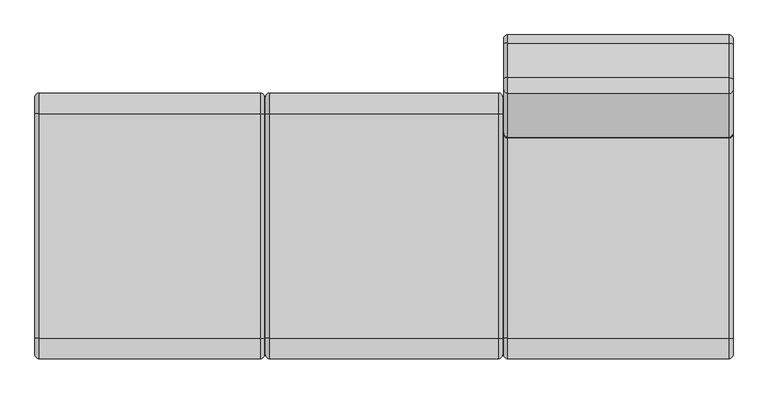
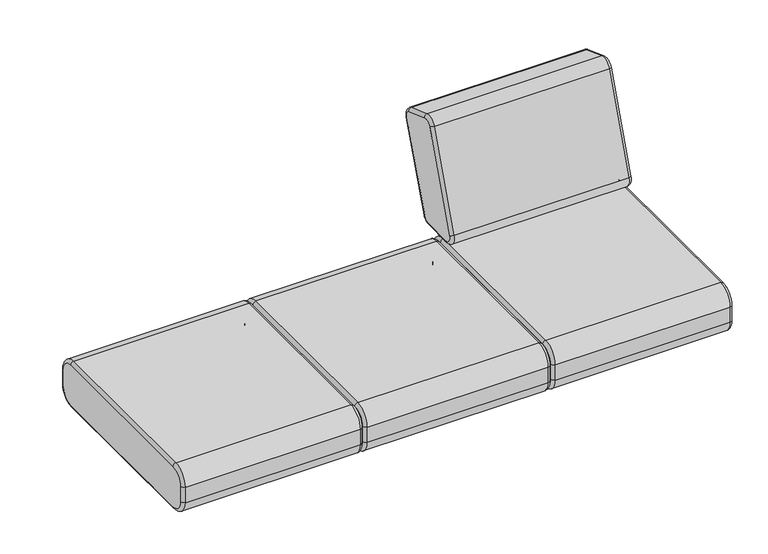
"""IFC4 building model written with IfcOpenShell, lengths in millimetres: furniture geometry."""

from ifc_helpers import new_model, si_unit, point, frame, origin, place, context, project, spatial, circle_curve, ellipse_curve, trimmed, source, transform, mapped, element, save
from ifc_brep_helpers import plane_surface, cylinder_surface, revolved_surface, advanced_brep


def furniture_29a9adb8(model_context):
    return source(origin(), model_context, "Body", "AdvancedBrep", [
        advanced_brep(
        [(-292.5, 542.7044583, 315.0), (-292.5, 582.7044583, 355.0), (-292.5, 582.7044583, 405.0), (-292.5, 542.7044583, 445.0), (-292.5, -5.0, 445.0), (-292.5, -45.0, 405.0), (-292.5, -45.0, 355.0), (-292.5, -5.0, 315.0), (-852.5, -5.0, 315.0), (-852.5, -45.0, 355.0), (-852.5, -45.0, 405.0), (-852.5, -5.0, 445.0), (-852.5, 542.7044583, 445.0), (-852.5, 582.7044583, 405.0), (-852.5, 582.7044583, 355.0), (-852.5, 542.7044583, 315.0), (-842.5, 592.7044583, 405.0), (-842.5, 542.7044583, 455.0), (-302.4999866, 542.7044583, 455.0), (-302.5, 592.7044583, 405.0), (-842.5, -5.0, 455.0), (-302.5, -5.0, 455.0), (-842.5, -55.0, 405.0), (-302.4999867, -55.0, 405.0), (-842.5, -55.0, 355.0), (-302.5, -55.0, 355.0), (-842.5, -5.0, 305.0), (-302.4999867, -5.0, 305.0), (-842.5, 542.7044583, 305.0), (-302.4999867, 542.7044583, 305.0), (-842.5, 592.7044583, 355.0), (-302.4999867, 592.7044583, 355.0)],
        [
            (0, 1, circle_curve(frame((-292.5, 542.7044583, 355.0), z_axis=(1.0, 0.0, 0.0), x_axis=(0.0, 0.0, -1.0)), 40.0)),
            (1, 2),
            (2, 3, circle_curve(frame((-292.5, 542.7044583, 405.0), z_axis=(1.0, 0.0, 0.0), x_axis=(0.0, 1.0, 0.0)), 40.0)),
            (3, 4),
            (4, 5, circle_curve(frame((-292.5, -5.0, 405.0), z_axis=(1.0, 0.0, 0.0), x_axis=(0.0, 0.0, 1.0)), 40.0)),
            (5, 6),
            (6, 7, circle_curve(frame((-292.5, -5.0, 355.0), z_axis=(1.0, 0.0, 0.0), x_axis=(0.0, -1.0, 0.0)), 40.0)),
            (7, 0),
            (8, 9, circle_curve(frame((-852.5, -5.0, 355.0), z_axis=(-1.0, 0.0, 0.0), x_axis=(0.0, 0.0, -1.0)), 40.0)),
            (9, 10),
            (10, 11, circle_curve(frame((-852.5, -5.0, 405.0), z_axis=(-1.0, 0.0, 0.0), x_axis=(0.0, -1.0, 0.0)), 40.0)),
            (11, 12),
            (12, 13, circle_curve(frame((-852.5, 542.7044583, 405.0), z_axis=(-1.0, 0.0, 0.0), x_axis=(0.0, 0.0, 1.0)), 40.0)),
            (13, 14),
            (14, 15, circle_curve(frame((-852.5, 542.7044583, 355.0), z_axis=(-1.0, 0.0, 0.0), x_axis=(0.0, 1.0, 0.0)), 40.0)),
            (15, 8),
            (16, 17, circle_curve(frame((-842.5, 542.7044583, 405.0), z_axis=(1.0, 0.0, 0.0), x_axis=(0.0, 1.0, 0.0)), 50.0)),
            (17, 18),
            (18, 19, circle_curve(frame((-302.5, 542.7044583, 405.0), z_axis=(-1.0, 0.0, 0.0), x_axis=(0.0, 1.0, 0.0)), 50.0)),
            (19, 16),
            (17, 20),
            (20, 21),
            (21, 18),
            (20, 22, circle_curve(frame((-842.5, -5.0, 405.0), z_axis=(1.0, 0.0, 0.0), x_axis=(0.0, 1.0, 0.0)), 50.0)),
            (22, 23),
            (23, 21, circle_curve(frame((-302.5, -5.0, 405.0), z_axis=(-1.0, 0.0, 0.0), x_axis=(0.0, 1.0, 0.0)), 50.0)),
            (22, 24),
            (24, 25),
            (25, 23),
            (24, 26, circle_curve(frame((-842.5, -5.0, 355.0), z_axis=(1.0, 0.0, 0.0), x_axis=(0.0, 1.0, 0.0)), 50.0)),
            (26, 27),
            (27, 25, circle_curve(frame((-302.5, -5.0, 355.0), z_axis=(-1.0, 0.0, 0.0), x_axis=(0.0, 1.0, 0.0)), 50.0)),
            (26, 28),
            (28, 29),
            (29, 27),
            (28, 30, circle_curve(frame((-842.5, 542.7044583, 355.0), z_axis=(1.0, 0.0, 0.0), x_axis=(0.0, 1.0, 0.0)), 50.0)),
            (30, 31),
            (31, 29, circle_curve(frame((-302.5, 542.7044583, 355.0), z_axis=(-1.0, 0.0, 0.0), x_axis=(0.0, 1.0, 0.0)), 50.0)),
            (30, 16),
            (19, 31),
            (24, 9, circle_curve(frame((-842.5, -45.0, 355.0), z_axis=(0.0, 0.0, -1.0), x_axis=(-1.0, 0.0, 0.0)), 10.0)),
            (8, 26, circle_curve(frame((-842.5, -5.0, 315.0), z_axis=(0.0, -1.0, 0.0), x_axis=(-1.0, 0.0, 0.0)), 10.0)),
            (22, 10, circle_curve(frame((-842.5, -45.0, 405.0), z_axis=(0.0, 0.0, -1.0), x_axis=(-1.0, 0.0, 0.0)), 10.0)),
            (20, 11, circle_curve(frame((-842.5, -5.0, 445.0), z_axis=(0.0, -1.0, 0.0), x_axis=(-1.0, 0.0, 0.0)), 10.0)),
            (17, 12, circle_curve(frame((-842.5, 542.7044583, 445.0), z_axis=(0.0, -1.0, 0.0), x_axis=(-1.0, 0.0, 0.0)), 10.0)),
            (16, 13, circle_curve(frame((-842.5, 582.7044583, 405.0), z_axis=(0.0, 0.0, 1.0), x_axis=(-1.0, 0.0, 0.0)), 10.0)),
            (30, 14, circle_curve(frame((-842.5, 582.7044583, 355.0), z_axis=(0.0, 0.0, 1.0), x_axis=(-1.0, 0.0, 0.0)), 10.0)),
            (28, 15, circle_curve(frame((-842.5, 542.7044583, 315.0), z_axis=(0.0, 1.0, 0.0), x_axis=(-1.0, 0.0, 0.0)), 10.0)),
            (31, 1, circle_curve(frame((-302.5, 582.7044583, 355.0), z_axis=(0.0, 0.0, -1.0), x_axis=(1.0, 0.0, 0.0)), 10.0)),
            (0, 29, circle_curve(frame((-302.5, 542.7044583, 315.0), z_axis=(0.0, 1.0, 0.0), x_axis=(1.0, 0.0, 0.0)), 10.0)),
            (19, 2, circle_curve(frame((-302.5, 582.7044583, 405.0), z_axis=(0.0, 0.0, -1.0), x_axis=(1.0, 0.0, 0.0)), 10.0)),
            (18, 3, circle_curve(frame((-302.5, 542.7044583, 445.0), z_axis=(0.0, 1.0, 0.0), x_axis=(1.0, 0.0, 0.0)), 10.0)),
            (21, 4, circle_curve(frame((-302.5, -5.0, 445.0), z_axis=(0.0, 1.0, 0.0), x_axis=(1.0, 0.0, 0.0)), 10.0)),
            (23, 5, circle_curve(frame((-302.5, -45.0, 405.0), z_axis=(0.0, 0.0, 1.0), x_axis=(1.0, 0.0, 0.0)), 10.0)),
            (25, 6, circle_curve(frame((-302.5, -45.0, 355.0), z_axis=(0.0, 0.0, 1.0), x_axis=(1.0, 0.0, 0.0)), 10.0)),
            (27, 7, circle_curve(frame((-302.5, -5.0, 315.0), z_axis=(0.0, -1.0, 0.0), x_axis=(1.0, 0.0, 0.0)), 10.0)),
        ],
        [
            plane_surface(frame((-292.5, 592.7044583, 405.0), z_axis=(1.0, 0.0, 0.0), x_axis=(0.0, 0.0, 1.0))),
            plane_surface(frame((-852.5, 592.7044583, 405.0), z_axis=(-1.0, 0.0, 0.0), x_axis=(0.0, 0.0, -1.0))),
            cylinder_surface(frame((-852.5, 542.7044583, 405.0), z_axis=(1.0, 0.0, 0.0), x_axis=(0.0, 1.0, 0.0)), 50.0),
            plane_surface(frame((-292.5, 542.7044583, 455.0), z_axis=(0.0, 0.0, 1.0), x_axis=(-1.0, 0.0, 0.0))),
            cylinder_surface(frame((-852.5, -5.0, 405.0), z_axis=(1.0, 0.0, 0.0), x_axis=(0.0, 1.0, 0.0)), 50.0),
            plane_surface(frame((-292.5, -55.0, 405.0), z_axis=(0.0, -1.0, 0.0), x_axis=(-1.0, 0.0, 0.0))),
            cylinder_surface(frame((-852.5, -5.0, 355.0), z_axis=(1.0, 0.0, 0.0), x_axis=(0.0, 1.0, 0.0)), 50.0),
            plane_surface(frame((-292.5, -5.0, 305.0), z_axis=(0.0, 0.0, -1.0), x_axis=(-1.0, 0.0, 0.0))),
            cylinder_surface(frame((-852.5, 542.7044583, 355.0), z_axis=(1.0, 0.0, 0.0), x_axis=(0.0, 1.0, 0.0)), 50.0),
            plane_surface(frame((-292.5, 592.7044583, 355.0), z_axis=(0.0, 1.0, 0.0), x_axis=(-1.0, 0.0, 0.0))),
            revolved_surface(trimmed(ellipse_curve(frame((-842.5, -5.0, 315.0), z_axis=(0.0, 1.0, 0.0), x_axis=(-1.0, 0.0, 0.0)), 10.0, 10.0), [point((-842.5, -5.0, 305.0))], [point((-852.5, -5.0, 315.0))], True, "CARTESIAN"), (-852.5, -5.0, 355.0), (-1.0, 0.0, 0.0)),
            cylinder_surface(frame((-842.5, -45.0, 355.0), z_axis=(0.0, 0.0, 1.0), x_axis=(-1.0, 0.0, 0.0)), 10.0),
            revolved_surface(trimmed(ellipse_curve(frame((-842.5, -45.0, 405.0), z_axis=(0.0, 0.0, -1.0), x_axis=(-1.0, 0.0, 0.0)), 10.0, 10.0), [point((-842.5, -55.0, 405.0))], [point((-852.5, -45.0, 405.0))], True, "CARTESIAN"), (-852.5, -5.0, 405.0), (-1.0, 0.0, 0.0)),
            cylinder_surface(frame((-842.5, -5.0, 445.0), z_axis=(0.0, 1.0, 0.0), x_axis=(-1.0, 0.0, 0.0)), 10.0),
            revolved_surface(trimmed(ellipse_curve(frame((-842.5, 542.7044583, 445.0), z_axis=(0.0, -1.0, 0.0), x_axis=(-1.0, 0.0, 0.0)), 10.0, 10.0), [point((-842.5, 542.7044583, 455.0))], [point((-852.5, 542.7044583, 445.0))], True, "CARTESIAN"), (-852.5, 542.7044583, 405.0), (-1.0, 0.0, 0.0)),
            cylinder_surface(frame((-842.5, 582.7044583, 405.0), z_axis=(0.0, 0.0, -1.0), x_axis=(-1.0, 0.0, 0.0)), 10.0),
            revolved_surface(trimmed(ellipse_curve(frame((-842.5, 582.7044583, 355.0), z_axis=(0.0, 0.0, 1.0), x_axis=(-1.0, 0.0, 0.0)), 10.0, 10.0), [point((-842.5, 592.7044583, 355.0))], [point((-852.5, 582.7044583, 355.0))], True, "CARTESIAN"), (-852.5, 542.7044583, 355.0), (-1.0, 0.0, 0.0)),
            cylinder_surface(frame((-842.5, 542.7044583, 315.0), z_axis=(0.0, -1.0, 0.0), x_axis=(-1.0, 0.0, 0.0)), 10.0),
            revolved_surface(trimmed(ellipse_curve(frame((-302.5, 542.7044583, 315.0), z_axis=(0.0, -1.0, 0.0), x_axis=(1.0, 0.0, 0.0)), 10.0, 10.0), [point((-302.5, 542.7044583, 305.0))], [point((-292.5, 542.7044583, 315.0))], True, "CARTESIAN"), (-292.5, 542.7044583, 355.0), (1.0, 0.0, 0.0)),
            cylinder_surface(frame((-302.5, 582.7044583, 355.0), z_axis=(0.0, 0.0, 1.0), x_axis=(1.0, 0.0, 0.0)), 10.0),
            revolved_surface(trimmed(ellipse_curve(frame((-302.5, 582.7044583, 405.0), z_axis=(0.0, 0.0, -1.0), x_axis=(1.0, 0.0, 0.0)), 10.0, 10.0), [point((-302.5, 592.7044583, 405.0))], [point((-292.5, 582.7044583, 405.0))], True, "CARTESIAN"), (-292.5, 542.7044583, 405.0), (1.0, 0.0, 0.0)),
            cylinder_surface(frame((-302.5, 542.7044583, 445.0), z_axis=(0.0, -1.0, 0.0), x_axis=(1.0, 0.0, 0.0)), 10.0),
            revolved_surface(trimmed(ellipse_curve(frame((-302.5, -5.0, 445.0), z_axis=(0.0, 1.0, 0.0), x_axis=(1.0, 0.0, 0.0)), 10.0, 10.0), [point((-302.5, -5.0, 455.0))], [point((-292.5, -5.0, 445.0))], True, "CARTESIAN"), (-292.5, -5.0, 405.0), (1.0, 0.0, 0.0)),
            cylinder_surface(frame((-302.5, -45.0, 405.0), z_axis=(0.0, 0.0, -1.0), x_axis=(1.0, 0.0, 0.0)), 10.0),
            revolved_surface(trimmed(ellipse_curve(frame((-302.5, -45.0, 355.0), z_axis=(0.0, 0.0, 1.0), x_axis=(1.0, 0.0, 0.0)), 10.0, 10.0), [point((-302.5, -55.0, 355.0))], [point((-292.5, -45.0, 355.0))], True, "CARTESIAN"), (-292.5, -5.0, 355.0), (1.0, 0.0, 0.0)),
            cylinder_surface(frame((-302.5, -5.0, 315.0), z_axis=(0.0, 1.0, 0.0), x_axis=(1.0, 0.0, 0.0)), 10.0),
        ],
        [
            (0, [[1, 2, 3, 4, 5, 6, 7, 8]]),
            (1, [[9, 10, 11, 12, 13, 14, 15, 16]]),
            (2, [[17, 18, 19, 20]]),
            (3, [[21, 22, 23, -18]]),
            (4, [[24, 25, 26, -22]]),
            (5, [[27, 28, 29, -25]]),
            (6, [[30, 31, 32, -28]]),
            (7, [[33, 34, 35, -31]]),
            (8, [[36, 37, 38, -34]]),
            (9, [[39, -20, 40, -37]]),
            (10, [[41, -9, 42, -30]]),
            (11, [[-41, -27, 43, -10]]),
            (12, [[-43, -24, 44, -11]]),
            (13, [[-44, -21, 45, -12]]),
            (14, [[-45, -17, 46, -13]]),
            (15, [[-46, -39, 47, -14]]),
            (16, [[-47, -36, 48, -15]]),
            (17, [[-42, -16, -48, -33]]),
            (18, [[49, -1, 50, -38]]),
            (19, [[-49, -40, 51, -2]]),
            (20, [[-51, -19, 52, -3]]),
            (21, [[-52, -23, 53, -4]]),
            (22, [[-53, -26, 54, -5]]),
            (23, [[-54, -29, 55, -6]]),
            (24, [[-55, -32, 56, -7]]),
            (25, [[-50, -8, -56, -35]]),
        ],
    ),
        advanced_brep(
        [(851.1853865, 609.5185405, 469.9348489), (851.1853865, 628.3736149, 483.1373142), (851.1853865, 723.5847628, 744.7277933), (851.1853865, 711.5923743, 770.4455535), (851.1853865, 627.0200384, 801.2273664), (851.1853865, 601.3022782, 789.2349779), (851.1853865, 494.8874666, 496.8626858), (851.1853865, 513.742541, 469.9348489), (291.1853865, 513.742541, 469.9348489), (291.1853865, 494.8874666, 496.8626858), (291.1853865, 601.3022782, 789.2349779), (291.1853865, 627.0200384, 801.2273664), (291.1853865, 711.5923743, 770.4455535), (291.1853865, 723.5847628, 744.7277933), (291.1853865, 628.3736149, 483.1373142), (291.1853865, 609.5185405, 469.9348489), (301.1853865, 630.4402399, 810.6242926), (301.1853865, 591.905352, 792.6551793), (841.1853984, 591.905352, 792.6551793), (841.1853865, 630.4402399, 810.6242926), (301.1853865, 485.4905403, 500.2828873), (841.1853865, 485.4905403, 500.2828873), (301.1853865, 513.742541, 459.9348489), (841.1853988, 513.742541, 459.9348489), (301.1853865, 609.5185405, 459.9348489), (841.1853987, 609.5185405, 459.9348489), (301.1853865, 637.7705411, 479.7171127), (841.1853987, 637.7705411, 479.7171127), (301.1853865, 732.9816891, 741.3075918), (841.1853865, 732.9816891, 741.3075918), (301.1853865, 715.0125757, 779.8424797), (841.1853984, 715.0125757, 779.8424797)],
        [
            (0, 1, circle_curve(frame((851.1853865, 609.5185405, 490.0), z_axis=(1.0, 0.0, 0.0), x_axis=(0.0, 0.0, -1.0)), 20.0651511)),
            (1, 2),
            (2, 3, circle_curve(frame((851.1853865, 704.7296884, 751.5904791), z_axis=(1.0, 0.0, 0.0), x_axis=(0.0, 0.9396926207859067, -0.3420201433256736)), 20.0651511)),
            (3, 4),
            (4, 5, circle_curve(frame((851.1853865, 620.1573526, 782.372292), z_axis=(1.0, 0.0, 0.0), x_axis=(0.0, 0.3420201433256753, 0.939692620785906)), 20.0651511)),
            (5, 6),
            (6, 7, circle_curve(frame((851.1853865, 513.742541, 490.0), z_axis=(1.0, 0.0, 0.0), x_axis=(0.0, -0.9396926207859095, 0.34202014332566555)), 20.0651511)),
            (7, 0),
            (8, 9, circle_curve(frame((291.1853865, 513.742541, 490.0), z_axis=(-1.0, 0.0, 0.0), x_axis=(0.0, 0.0, -1.0)), 20.0651511)),
            (9, 10),
            (10, 11, circle_curve(frame((291.1853865, 620.1573526, 782.372292), z_axis=(-1.0, 0.0, 0.0), x_axis=(0.0, -0.9396926207859101, 0.34202014332566405)), 20.0651511)),
            (11, 12),
            (12, 13, circle_curve(frame((291.1853865, 704.7296884, 751.5904791), z_axis=(-1.0, 0.0, 0.0), x_axis=(0.0, 0.34202014332566566, 0.9396926207859095)), 20.0651511)),
            (13, 14),
            (14, 15, circle_curve(frame((291.1853865, 609.5185405, 490.0), z_axis=(-1.0, 0.0, 0.0), x_axis=(0.0, 0.9396926207859108, -0.3420201433256623)), 20.0651511)),
            (15, 8),
            (16, 17, circle_curve(frame((301.1853865, 620.1573526, 782.372292), z_axis=(1.0, 0.0, 0.0), x_axis=(0.0, 1.0, 0.0)), 30.0651511)),
            (17, 18),
            (18, 19, circle_curve(frame((841.1853865, 620.1573526, 782.372292), z_axis=(-1.0, 0.0, 0.0), x_axis=(0.0, 1.0, 0.0)), 30.0651511)),
            (19, 16),
            (17, 20),
            (20, 21),
            (21, 18),
            (20, 22, circle_curve(frame((301.1853865, 513.742541, 490.0), z_axis=(1.0, 0.0, 0.0), x_axis=(0.0, 1.0, 0.0)), 30.0651511)),
            (22, 23),
            (23, 21, circle_curve(frame((841.1853865, 513.742541, 490.0), z_axis=(-1.0, 0.0, 0.0), x_axis=(0.0, 1.0, 0.0)), 30.0651511)),
            (22, 24),
            (24, 25),
            (25, 23),
            (24, 26, circle_curve(frame((301.1853865, 609.5185405, 490.0), z_axis=(1.0, 0.0, 0.0), x_axis=(0.0, 1.0, 0.0)), 30.0651511)),
            (26, 27),
            (27, 25, circle_curve(frame((841.1853865, 609.5185405, 490.0), z_axis=(-1.0, 0.0, 0.0), x_axis=(0.0, 1.0, 0.0)), 30.0651511)),
            (26, 28),
            (28, 29),
            (29, 27),
            (28, 30, circle_curve(frame((301.1853865, 704.7296884, 751.5904791), z_axis=(1.0, 0.0, 0.0), x_axis=(0.0, 1.0, 0.0)), 30.0651511)),
            (30, 31),
            (31, 29, circle_curve(frame((841.1853865, 704.7296884, 751.5904791), z_axis=(-1.0, 0.0, 0.0), x_axis=(0.0, 1.0, 0.0)), 30.0651511)),
            (30, 16),
            (19, 31),
            (20, 9, circle_curve(frame((301.1853865, 494.8874666, 496.8626858), z_axis=(0.0, -0.34202014332566616, -0.9396926207859093), x_axis=(-1.0, 0.0, 0.0)), 10.0)),
            (8, 22, circle_curve(frame((301.1853865, 513.742541, 469.9348489), z_axis=(0.0, -1.0, 0.0), x_axis=(-1.0, 0.0, 0.0)), 10.0)),
            (17, 10, circle_curve(frame((301.1853865, 601.3022782, 789.2349779), z_axis=(0.0, -0.3420201433256583, -0.9396926207859122), x_axis=(-1.0, 0.0, 0.0)), 10.0)),
            (16, 11, circle_curve(frame((301.1853865, 627.0200384, 801.2273664), z_axis=(0.0, -0.9396926207859073, 0.34202014332567154), x_axis=(-1.0, 0.0, 0.0)), 10.0)),
            (30, 12, circle_curve(frame((301.1853865, 711.5923743, 770.4455535), z_axis=(0.0, -0.9396926207859225, 0.34202014332562997), x_axis=(-1.0, 0.0, 0.0)), 10.0)),
            (28, 13, circle_curve(frame((301.1853865, 723.5847628, 744.7277933), z_axis=(0.0, 0.34202014332567504, 0.9396926207859061), x_axis=(-1.0, 0.0, 0.0)), 10.0)),
            (26, 14, circle_curve(frame((301.1853865, 628.3736149, 483.1373142), z_axis=(0.0, 0.34202014332565633, 0.939692620785913), x_axis=(-1.0, 0.0, 0.0)), 10.0)),
            (24, 15, circle_curve(frame((301.1853865, 609.5185405, 469.9348489), z_axis=(0.0, 0.9999999999999999, 0.0), x_axis=(-1.0, 0.0, 0.0)), 10.0)),
            (27, 1, circle_curve(frame((841.1853865, 628.3736149, 483.1373142), z_axis=(0.0, -0.3420201433256674, -0.9396926207859089), x_axis=(1.0, 0.0, 0.0)), 10.0)),
            (0, 25, circle_curve(frame((841.1853865, 609.5185405, 469.9348489), z_axis=(0.0, 1.0, 0.0), x_axis=(1.0, 0.0, 0.0)), 10.0)),
            (29, 2, circle_curve(frame((841.1853865, 723.5847628, 744.7277933), z_axis=(0.0, -0.34202014332565644, -0.9396926207859129), x_axis=(1.0, 0.0, 0.0)), 10.0)),
            (31, 3, circle_curve(frame((841.1853865, 711.5923743, 770.4455535), z_axis=(0.0, 0.9396926207859082, -0.3420201433256694), x_axis=(1.0, 0.0, 0.0)), 10.0)),
            (19, 4, circle_curve(frame((841.1853865, 627.0200384, 801.2273664), z_axis=(0.0, 0.9396926207859224, -0.3420201433256302), x_axis=(1.0, 0.0, 0.0)), 10.0)),
            (18, 5, circle_curve(frame((841.1853865, 601.3022782, 789.2349779), z_axis=(0.0, 0.34202014332566893, 0.9396926207859083), x_axis=(1.0, 0.0, 0.0)), 10.0)),
            (21, 6, circle_curve(frame((841.1853865, 494.8874666, 496.8626858), z_axis=(0.0, 0.3420201433256585, 0.9396926207859122), x_axis=(1.0, 0.0, 0.0)), 10.0)),
            (23, 7, circle_curve(frame((841.1853865, 513.742541, 469.9348489), z_axis=(0.0, -1.0, 0.0), x_axis=(1.0, 0.0, 0.0)), 10.0)),
        ],
        [
            plane_surface(frame((851.1853865, 650.2225036, 782.372292), z_axis=(1.0, 0.0, 0.0), x_axis=(0.0, 0.0, 1.0))),
            plane_surface(frame((291.1853865, 650.2225036, 782.372292), z_axis=(-1.0, 0.0, 0.0), x_axis=(0.0, 0.0, -1.0))),
            cylinder_surface(frame((291.1853865, 620.1573526, 782.372292), z_axis=(1.0, 0.0, 0.0), x_axis=(0.0, 1.0, 0.0)), 30.0651511),
            plane_surface(frame((851.1853865, 591.905352, 792.6551793), z_axis=(0.0, -0.9396926207859123, 0.3420201433256582), x_axis=(-1.0, 0.0, 0.0))),
            cylinder_surface(frame((291.1853865, 513.742541, 490.0), z_axis=(1.0, 0.0, 0.0), x_axis=(0.0, 1.0, 0.0)), 30.0651511),
            plane_surface(frame((851.1853865, 513.742541, 459.9348489), z_axis=(0.0, 0.0, -1.0), x_axis=(-1.0, 0.0, 0.0))),
            cylinder_surface(frame((291.1853865, 609.5185405, 490.0), z_axis=(1.0, 0.0, 0.0), x_axis=(0.0, 1.0, 0.0)), 30.0651511),
            plane_surface(frame((851.1853865, 637.7705411, 479.7171127), z_axis=(0.0, 0.9396926207859131, -0.3420201433256561), x_axis=(-1.0, 0.0, 0.0))),
            cylinder_surface(frame((291.1853865, 704.7296884, 751.5904791), z_axis=(1.0, 0.0, 0.0), x_axis=(0.0, 1.0, 0.0)), 30.0651511),
            plane_surface(frame((851.1853865, 715.0125757, 779.8424797), z_axis=(0.0, 0.34202014332562986, 0.9396926207859226), x_axis=(-1.0, 0.0, 0.0))),
            revolved_surface(trimmed(ellipse_curve(frame((301.1853865, 513.742541, 469.9348489), z_axis=(0.0, 1.0, 0.0), x_axis=(-1.0, 0.0, 0.0)), 10.0, 10.0), [point((301.1853865, 513.742541, 459.9348489))], [point((291.1853865, 513.742541, 469.9348489))], True, "CARTESIAN"), (291.1853865, 513.742541, 490.0), (-1.0, 0.0, 0.0)),
            cylinder_surface(frame((301.1853865, 494.8874666, 496.8626858), z_axis=(0.0, 0.3420201433256583, 0.9396926207859122), x_axis=(-1.0, 0.0, 0.0)), 10.0),
            revolved_surface(trimmed(ellipse_curve(frame((301.1853865, 601.3022782, 789.2349779), z_axis=(0.0, -0.3420201433256641, -0.9396926207859101), x_axis=(-1.0, 0.0, 0.0)), 10.0, 10.0), [point((301.1853865, 591.905352, 792.6551793))], [point((291.1853865, 601.3022782, 789.2349779))], True, "CARTESIAN"), (291.1853865, 620.1573526, 782.372292), (-1.0, 0.0, 0.0)),
            cylinder_surface(frame((301.1853865, 627.0200384, 801.2273664), z_axis=(0.0, 0.9396926207859225, -0.34202014332562997), x_axis=(-1.0, 0.0, 0.0)), 10.0),
            revolved_surface(trimmed(ellipse_curve(frame((301.1853865, 711.5923743, 770.4455535), z_axis=(0.0, -0.9396926207859094, 0.34202014332566594), x_axis=(-1.0, 0.0, 0.0)), 10.0, 10.0), [point((301.1853865, 715.0125757, 779.8424797))], [point((291.1853865, 711.5923743, 770.4455535))], True, "CARTESIAN"), (291.1853865, 704.7296884, 751.5904791), (-1.0, 0.0, 0.0)),
            cylinder_surface(frame((301.1853865, 723.5847628, 744.7277933), z_axis=(0.0, -0.34202014332565633, -0.939692620785913), x_axis=(-1.0, 0.0, 0.0)), 10.0),
            revolved_surface(trimmed(ellipse_curve(frame((301.1853865, 628.3736149, 483.1373142), z_axis=(0.0, 0.3420201433256624, 0.9396926207859108), x_axis=(-1.0, 0.0, 0.0)), 10.0, 10.0), [point((301.1853865, 637.7705411, 479.7171127))], [point((291.1853865, 628.3736149, 483.1373142))], True, "CARTESIAN"), (291.1853865, 609.5185405, 490.0), (-1.0, 0.0, 0.0)),
            cylinder_surface(frame((301.1853865, 609.5185405, 469.9348489), z_axis=(0.0, -1.0, 0.0), x_axis=(-1.0, 0.0, 0.0)), 10.0),
            revolved_surface(trimmed(ellipse_curve(frame((841.1853865, 609.5185405, 469.9348489), z_axis=(0.0, -1.0, 0.0), x_axis=(1.0, 0.0, 0.0)), 10.0, 10.0), [point((841.1853865, 609.5185405, 459.9348489))], [point((851.1853865, 609.5185405, 469.9348489))], True, "CARTESIAN"), (851.1853865, 609.5185405, 490.0), (1.0, 0.0, 0.0)),
            cylinder_surface(frame((841.1853865, 628.3736149, 483.1373142), z_axis=(0.0, 0.34202014332565644, 0.9396926207859129), x_axis=(1.0, 0.0, 0.0)), 10.0),
            revolved_surface(trimmed(ellipse_curve(frame((841.1853865, 723.5847628, 744.7277933), z_axis=(0.0, -0.34202014332567393, -0.9396926207859065), x_axis=(1.0, 0.0, 0.0)), 10.0, 10.0), [point((841.1853865, 732.9816891, 741.3075918))], [point((851.1853865, 723.5847628, 744.7277933))], True, "CARTESIAN"), (851.1853865, 704.7296884, 751.5904791), (1.0, 0.0, 0.0)),
            cylinder_surface(frame((841.1853865, 711.5923743, 770.4455535), z_axis=(0.0, -0.9396926207859224, 0.3420201433256302), x_axis=(1.0, 0.0, 0.0)), 10.0),
            revolved_surface(trimmed(ellipse_curve(frame((841.1853865, 627.0200384, 801.2273664), z_axis=(0.0, 0.9396926207859059, -0.3420201433256756), x_axis=(1.0, 0.0, 0.0)), 10.0, 10.0), [point((841.1853865, 630.4402399, 810.6242926))], [point((851.1853865, 627.0200384, 801.2273664))], True, "CARTESIAN"), (851.1853865, 620.1573526, 782.372292), (1.0, 0.0, 0.0)),
            cylinder_surface(frame((841.1853865, 601.3022782, 789.2349779), z_axis=(0.0, -0.3420201433256585, -0.9396926207859122), x_axis=(1.0, 0.0, 0.0)), 10.0),
            revolved_surface(trimmed(ellipse_curve(frame((841.1853865, 494.8874666, 496.8626858), z_axis=(0.0, 0.34202014332566594, 0.9396926207859094), x_axis=(1.0, 0.0, 0.0)), 10.0, 10.0), [point((841.1853865, 485.4905403, 500.2828873))], [point((851.1853865, 494.8874666, 496.8626858))], True, "CARTESIAN"), (851.1853865, 513.742541, 490.0), (1.0, 0.0, 0.0)),
            cylinder_surface(frame((841.1853865, 513.742541, 469.9348489), z_axis=(0.0, 1.0, 0.0), x_axis=(1.0, 0.0, 0.0)), 10.0),
        ],
        [
            (0, [[1, 2, 3, 4, 5, 6, 7, 8]]),
            (1, [[9, 10, 11, 12, 13, 14, 15, 16]]),
            (2, [[17, 18, 19, 20]]),
            (3, [[21, 22, 23, -18]]),
            (4, [[24, 25, 26, -22]]),
            (5, [[27, 28, 29, -25]]),
            (6, [[30, 31, 32, -28]]),
            (7, [[33, 34, 35, -31]]),
            (8, [[36, 37, 38, -34]]),
            (9, [[39, -20, 40, -37]]),
            (10, [[41, -9, 42, -24]]),
            (11, [[-41, -21, 43, -10]]),
            (12, [[-43, -17, 44, -11]]),
            (13, [[-44, -39, 45, -12]]),
            (14, [[-45, -36, 46, -13]]),
            (15, [[-46, -33, 47, -14]]),
            (16, [[-47, -30, 48, -15]]),
            (17, [[-42, -16, -48, -27]]),
            (18, [[49, -1, 50, -32]]),
            (19, [[-49, -35, 51, -2]]),
            (20, [[-51, -38, 52, -3]]),
            (21, [[-52, -40, 53, -4]]),
            (22, [[-53, -19, 54, -5]]),
            (23, [[-54, -23, 55, -6]]),
            (24, [[-55, -26, 56, -7]]),
            (25, [[-50, -8, -56, -29]]),
        ],
    ),
        advanced_brep(
        [(851.1853865, 542.7044583, 315.0), (851.1853865, 582.7044583, 355.0), (851.1853865, 582.7044583, 405.0), (851.1853865, 542.7044583, 445.0), (851.1853865, -5.0, 445.0), (851.1853865, -45.0, 405.0), (851.1853865, -45.0, 355.0), (851.1853865, -5.0, 315.0), (291.1853865, -5.0, 315.0), (291.1853865, -45.0, 355.0), (291.1853865, -45.0, 405.0), (291.1853865, -5.0, 445.0), (291.1853865, 542.7044583, 445.0), (291.1853865, 582.7044583, 405.0), (291.1853865, 582.7044583, 355.0), (291.1853865, 542.7044583, 315.0), (301.1853865, 592.7044583, 405.0), (301.1853865, 542.7044583, 455.0), (841.1854, 542.7044583, 455.0), (841.1853865, 592.7044583, 405.0), (301.1853865, -5.0, 455.0), (841.1853865, -5.0, 455.0), (301.1853865, -55.0, 405.0), (841.1854, -55.0, 405.0), (301.1853865, -55.0, 355.0), (841.1853865, -55.0, 355.0), (301.1853865, -5.0, 305.0), (841.1853999, -5.0, 305.0), (301.1853865, 542.7044583, 305.0), (841.1854, 542.7044583, 305.0), (301.1853865, 592.7044583, 355.0), (841.1854, 592.7044583, 355.0)],
        [
            (0, 1, circle_curve(frame((851.1853865, 542.7044583, 355.0), z_axis=(1.0, 0.0, 0.0), x_axis=(0.0, 0.0, -1.0)), 40.0)),
            (1, 2),
            (2, 3, circle_curve(frame((851.1853865, 542.7044583, 405.0), z_axis=(1.0, 0.0, 0.0), x_axis=(0.0, 1.0, 0.0)), 40.0)),
            (3, 4),
            (4, 5, circle_curve(frame((851.1853865, -5.0, 405.0), z_axis=(1.0, 0.0, 0.0), x_axis=(0.0, 0.0, 1.0)), 40.0)),
            (5, 6),
            (6, 7, circle_curve(frame((851.1853865, -5.0, 355.0), z_axis=(1.0, 0.0, 0.0), x_axis=(0.0, -1.0, 0.0)), 40.0)),
            (7, 0),
            (8, 9, circle_curve(frame((291.1853865, -5.0, 355.0), z_axis=(-1.0, 0.0, 0.0), x_axis=(0.0, 0.0, -1.0)), 40.0)),
            (9, 10),
            (10, 11, circle_curve(frame((291.1853865, -5.0, 405.0), z_axis=(-1.0, 0.0, 0.0), x_axis=(0.0, -1.0, 0.0)), 40.0)),
            (11, 12),
            (12, 13, circle_curve(frame((291.1853865, 542.7044583, 405.0), z_axis=(-1.0, 0.0, 0.0), x_axis=(0.0, 0.0, 1.0)), 40.0)),
            (13, 14),
            (14, 15, circle_curve(frame((291.1853865, 542.7044583, 355.0), z_axis=(-1.0, 0.0, 0.0), x_axis=(0.0, 1.0, 0.0)), 40.0)),
            (15, 8),
            (16, 17, circle_curve(frame((301.1853865, 542.7044583, 405.0), z_axis=(1.0, 0.0, 0.0), x_axis=(0.0, 1.0, 0.0)), 50.0)),
            (17, 18),
            (18, 19, circle_curve(frame((841.1853865, 542.7044583, 405.0), z_axis=(-1.0, 0.0, 0.0), x_axis=(0.0, 1.0, 0.0)), 50.0)),
            (19, 16),
            (17, 20),
            (20, 21),
            (21, 18),
            (20, 22, circle_curve(frame((301.1853865, -5.0, 405.0), z_axis=(1.0, 0.0, 0.0), x_axis=(0.0, 1.0, 0.0)), 50.0)),
            (22, 23),
            (23, 21, circle_curve(frame((841.1853865, -5.0, 405.0), z_axis=(-1.0, 0.0, 0.0), x_axis=(0.0, 1.0, 0.0)), 50.0)),
            (22, 24),
            (24, 25),
            (25, 23),
            (24, 26, circle_curve(frame((301.1853865, -5.0, 355.0), z_axis=(1.0, 0.0, 0.0), x_axis=(0.0, 1.0, 0.0)), 50.0)),
            (26, 27),
            (27, 25, circle_curve(frame((841.1853865, -5.0, 355.0), z_axis=(-1.0, 0.0, 0.0), x_axis=(0.0, 1.0, 0.0)), 50.0)),
            (26, 28),
            (28, 29),
            (29, 27),
            (28, 30, circle_curve(frame((301.1853865, 542.7044583, 355.0), z_axis=(1.0, 0.0, 0.0), x_axis=(0.0, 1.0, 0.0)), 50.0)),
            (30, 31),
            (31, 29, circle_curve(frame((841.1853865, 542.7044583, 355.0), z_axis=(-1.0, 0.0, 0.0), x_axis=(0.0, 1.0, 0.0)), 50.0)),
            (30, 16),
            (19, 31),
            (24, 9, circle_curve(frame((301.1853865, -45.0, 355.0), z_axis=(0.0, 0.0, -1.0), x_axis=(-1.0, 0.0, 0.0)), 10.0)),
            (8, 26, circle_curve(frame((301.1853865, -5.0, 315.0), z_axis=(0.0, -1.0, 0.0), x_axis=(-1.0, 0.0, 0.0)), 10.0)),
            (22, 10, circle_curve(frame((301.1853865, -45.0, 405.0), z_axis=(0.0, 0.0, -1.0), x_axis=(-1.0, 0.0, 0.0)), 10.0)),
            (20, 11, circle_curve(frame((301.1853865, -5.0, 445.0), z_axis=(0.0, -1.0, 0.0), x_axis=(-1.0, 0.0, 0.0)), 10.0)),
            (17, 12, circle_curve(frame((301.1853865, 542.7044583, 445.0), z_axis=(0.0, -1.0, 0.0), x_axis=(-1.0, 0.0, 0.0)), 10.0)),
            (16, 13, circle_curve(frame((301.1853865, 582.7044583, 405.0), z_axis=(0.0, 0.0, 1.0), x_axis=(-1.0, 0.0, 0.0)), 10.0)),
            (30, 14, circle_curve(frame((301.1853865, 582.7044583, 355.0), z_axis=(0.0, 0.0, 1.0), x_axis=(-1.0, 0.0, 0.0)), 10.0)),
            (28, 15, circle_curve(frame((301.1853865, 542.7044583, 315.0), z_axis=(0.0, 1.0, 0.0), x_axis=(-1.0, 0.0, 0.0)), 10.0)),
            (31, 1, circle_curve(frame((841.1853865, 582.7044583, 355.0), z_axis=(0.0, 0.0, -1.0), x_axis=(1.0, 0.0, 0.0)), 10.0)),
            (0, 29, circle_curve(frame((841.1853865, 542.7044583, 315.0), z_axis=(0.0, 1.0, 0.0), x_axis=(1.0, 0.0, 0.0)), 10.0)),
            (19, 2, circle_curve(frame((841.1853865, 582.7044583, 405.0), z_axis=(0.0, 0.0, -1.0), x_axis=(1.0, 0.0, 0.0)), 10.0)),
            (18, 3, circle_curve(frame((841.1853865, 542.7044583, 445.0), z_axis=(0.0, 1.0, 0.0), x_axis=(1.0, 0.0, 0.0)), 10.0)),
            (21, 4, circle_curve(frame((841.1853865, -5.0, 445.0), z_axis=(0.0, 1.0, 0.0), x_axis=(1.0, 0.0, 0.0)), 10.0)),
            (23, 5, circle_curve(frame((841.1853865, -45.0, 405.0), z_axis=(0.0, 0.0, 1.0), x_axis=(1.0, 0.0, 0.0)), 10.0)),
            (25, 6, circle_curve(frame((841.1853865, -45.0, 355.0), z_axis=(0.0, 0.0, 1.0), x_axis=(1.0, 0.0, 0.0)), 10.0)),
            (27, 7, circle_curve(frame((841.1853865, -5.0, 315.0), z_axis=(0.0, -1.0, 0.0), x_axis=(1.0, 0.0, 0.0)), 10.0)),
        ],
        [
            plane_surface(frame((851.1853865, 592.7044583, 405.0), z_axis=(1.0, 0.0, 0.0), x_axis=(0.0, 0.0, 1.0))),
            plane_surface(frame((291.1853865, 592.7044583, 405.0), z_axis=(-1.0, 0.0, 0.0), x_axis=(0.0, 0.0, -1.0))),
            cylinder_surface(frame((291.1853865, 542.7044583, 405.0), z_axis=(1.0, 0.0, 0.0), x_axis=(0.0, 1.0, 0.0)), 50.0),
            plane_surface(frame((851.1853865, 542.7044583, 455.0), z_axis=(0.0, 0.0, 1.0), x_axis=(-1.0, 0.0, 0.0))),
            cylinder_surface(frame((291.1853865, -5.0, 405.0), z_axis=(1.0, 0.0, 0.0), x_axis=(0.0, 1.0, 0.0)), 50.0),
            plane_surface(frame((851.1853865, -55.0, 405.0), z_axis=(0.0, -1.0, 0.0), x_axis=(-1.0, 0.0, 0.0))),
            cylinder_surface(frame((291.1853865, -5.0, 355.0), z_axis=(1.0, 0.0, 0.0), x_axis=(0.0, 1.0, 0.0)), 50.0),
            plane_surface(frame((851.1853865, -5.0, 305.0), z_axis=(0.0, 0.0, -1.0), x_axis=(-1.0, 0.0, 0.0))),
            cylinder_surface(frame((291.1853865, 542.7044583, 355.0), z_axis=(1.0, 0.0, 0.0), x_axis=(0.0, 1.0, 0.0)), 50.0),
            plane_surface(frame((851.1853865, 592.7044583, 355.0), z_axis=(0.0, 1.0, 0.0), x_axis=(-1.0, 0.0, 0.0))),
            revolved_surface(trimmed(ellipse_curve(frame((301.1853865, -5.0, 315.0), z_axis=(0.0, 1.0, 0.0), x_axis=(-1.0, 0.0, 0.0)), 10.0, 10.0), [point((301.1853865, -5.0, 305.0))], [point((291.1853865, -5.0, 315.0))], True, "CARTESIAN"), (291.1853865, -5.0, 355.0), (-1.0, 0.0, 0.0)),
            cylinder_surface(frame((301.1853865, -45.0, 355.0), z_axis=(0.0, 0.0, 1.0), x_axis=(-1.0, 0.0, 0.0)), 10.0),
            revolved_surface(trimmed(ellipse_curve(frame((301.1853865, -45.0, 405.0), z_axis=(0.0, 0.0, -1.0), x_axis=(-1.0, 0.0, 0.0)), 10.0, 10.0), [point((301.1853865, -55.0, 405.0))], [point((291.1853865, -45.0, 405.0))], True, "CARTESIAN"), (291.1853865, -5.0, 405.0), (-1.0, 0.0, 0.0)),
            cylinder_surface(frame((301.1853865, -5.0, 445.0), z_axis=(0.0, 1.0, 0.0), x_axis=(-1.0, 0.0, 0.0)), 10.0),
            revolved_surface(trimmed(ellipse_curve(frame((301.1853865, 542.7044583, 445.0), z_axis=(0.0, -1.0, 0.0), x_axis=(-1.0, 0.0, 0.0)), 10.0, 10.0), [point((301.1853865, 542.7044583, 455.0))], [point((291.1853865, 542.7044583, 445.0))], True, "CARTESIAN"), (291.1853865, 542.7044583, 405.0), (-1.0, 0.0, 0.0)),
            cylinder_surface(frame((301.1853865, 582.7044583, 405.0), z_axis=(0.0, 0.0, -1.0), x_axis=(-1.0, 0.0, 0.0)), 10.0),
            revolved_surface(trimmed(ellipse_curve(frame((301.1853865, 582.7044583, 355.0), z_axis=(0.0, 0.0, 1.0), x_axis=(-1.0, 0.0, 0.0)), 10.0, 10.0), [point((301.1853865, 592.7044583, 355.0))], [point((291.1853865, 582.7044583, 355.0))], True, "CARTESIAN"), (291.1853865, 542.7044583, 355.0), (-1.0, 0.0, 0.0)),
            cylinder_surface(frame((301.1853865, 542.7044583, 315.0), z_axis=(0.0, -1.0, 0.0), x_axis=(-1.0, 0.0, 0.0)), 10.0),
            revolved_surface(trimmed(ellipse_curve(frame((841.1853865, 542.7044583, 315.0), z_axis=(0.0, -1.0, 0.0), x_axis=(1.0, 0.0, 0.0)), 10.0, 10.0), [point((841.1853865, 542.7044583, 305.0))], [point((851.1853865, 542.7044583, 315.0))], True, "CARTESIAN"), (851.1853865, 542.7044583, 355.0), (1.0, 0.0, 0.0)),
            cylinder_surface(frame((841.1853865, 582.7044583, 355.0), z_axis=(0.0, 0.0, 1.0), x_axis=(1.0, 0.0, 0.0)), 10.0),
            revolved_surface(trimmed(ellipse_curve(frame((841.1853865, 582.7044583, 405.0), z_axis=(0.0, 0.0, -1.0), x_axis=(1.0, 0.0, 0.0)), 10.0, 10.0), [point((841.1853865, 592.7044583, 405.0))], [point((851.1853865, 582.7044583, 405.0))], True, "CARTESIAN"), (851.1853865, 542.7044583, 405.0), (1.0, 0.0, 0.0)),
            cylinder_surface(frame((841.1853865, 542.7044583, 445.0), z_axis=(0.0, -1.0, 0.0), x_axis=(1.0, 0.0, 0.0)), 10.0),
            revolved_surface(trimmed(ellipse_curve(frame((841.1853865, -5.0, 445.0), z_axis=(0.0, 1.0, 0.0), x_axis=(1.0, 0.0, 0.0)), 10.0, 10.0), [point((841.1853865, -5.0, 455.0))], [point((851.1853865, -5.0, 445.0))], True, "CARTESIAN"), (851.1853865, -5.0, 405.0), (1.0, 0.0, 0.0)),
            cylinder_surface(frame((841.1853865, -45.0, 405.0), z_axis=(0.0, 0.0, -1.0), x_axis=(1.0, 0.0, 0.0)), 10.0),
            revolved_surface(trimmed(ellipse_curve(frame((841.1853865, -45.0, 355.0), z_axis=(0.0, 0.0, 1.0), x_axis=(1.0, 0.0, 0.0)), 10.0, 10.0), [point((841.1853865, -55.0, 355.0))], [point((851.1853865, -45.0, 355.0))], True, "CARTESIAN"), (851.1853865, -5.0, 355.0), (1.0, 0.0, 0.0)),
            cylinder_surface(frame((841.1853865, -5.0, 315.0), z_axis=(0.0, 1.0, 0.0), x_axis=(1.0, 0.0, 0.0)), 10.0),
        ],
        [
            (0, [[1, 2, 3, 4, 5, 6, 7, 8]]),
            (1, [[9, 10, 11, 12, 13, 14, 15, 16]]),
            (2, [[17, 18, 19, 20]]),
            (3, [[21, 22, 23, -18]]),
            (4, [[24, 25, 26, -22]]),
            (5, [[27, 28, 29, -25]]),
            (6, [[30, 31, 32, -28]]),
            (7, [[33, 34, 35, -31]]),
            (8, [[36, 37, 38, -34]]),
            (9, [[39, -20, 40, -37]]),
            (10, [[41, -9, 42, -30]]),
            (11, [[-41, -27, 43, -10]]),
            (12, [[-43, -24, 44, -11]]),
            (13, [[-44, -21, 45, -12]]),
            (14, [[-45, -17, 46, -13]]),
            (15, [[-46, -39, 47, -14]]),
            (16, [[-47, -36, 48, -15]]),
            (17, [[-42, -16, -48, -33]]),
            (18, [[49, -1, 50, -38]]),
            (19, [[-49, -40, 51, -2]]),
            (20, [[-51, -19, 52, -3]]),
            (21, [[-52, -23, 53, -4]]),
            (22, [[-53, -26, 54, -5]]),
            (23, [[-54, -29, 55, -6]]),
            (24, [[-55, -32, 56, -7]]),
            (25, [[-50, -8, -56, -35]]),
        ],
    ),
        advanced_brep(
        [(288.5853906, 542.7044583, 315.0), (288.5853906, 582.7044583, 355.0), (288.5853906, 582.7044583, 405.0), (288.5853906, 542.7044583, 445.0), (288.5853906, -5.0, 445.0), (288.5853906, -45.0, 405.0), (288.5853906, -45.0, 355.0), (288.5853906, -5.0, 315.0), (-290.0, 542.7044583, 445.0), (-290.0, 582.7044583, 405.0), (-290.0, 582.7044583, 355.0), (-290.0, 542.7044583, 315.0), (-290.0, -5.0, 315.0), (-290.0, -45.0, 355.0), (-290.0, -45.0, 405.0), (-290.0, -5.0, 445.0), (-280.0, 592.7044583, 405.0), (-280.0, 542.7044583, 455.0), (278.585404, 542.7044583, 455.0), (278.5853906, 592.7044583, 405.0), (-280.0, -5.0, 455.0), (278.5853906, -5.0, 455.0), (-280.0, -55.0, 405.0), (278.585404, -55.0, 405.0), (-280.0, -55.0, 355.0), (278.5853906, -55.0, 355.0), (-280.0, -5.0, 305.0), (278.585404, -5.0, 305.0), (-280.0, 542.7044583, 305.0), (278.585404, 542.7044583, 305.0), (-280.0, 592.7044583, 355.0), (278.585404, 592.7044583, 355.0)],
        [
            (0, 1, circle_curve(frame((288.5853906, 542.7044583, 355.0), z_axis=(1.0, 0.0, 0.0), x_axis=(0.0, 0.0, -1.0)), 40.0)),
            (1, 2),
            (2, 3, circle_curve(frame((288.5853906, 542.7044583, 405.0), z_axis=(1.0, 0.0, 0.0), x_axis=(0.0, 1.0, 0.0)), 40.0)),
            (3, 4),
            (4, 5, circle_curve(frame((288.5853906, -5.0, 405.0), z_axis=(1.0, 0.0, 0.0), x_axis=(0.0, 0.0, 1.0)), 40.0)),
            (5, 6),
            (6, 7, circle_curve(frame((288.5853906, -5.0, 355.0), z_axis=(1.0, 0.0, 0.0), x_axis=(0.0, -1.0, 0.0)), 40.0)),
            (7, 0),
            (8, 9, circle_curve(frame((-290.0, 542.7044583, 405.0), z_axis=(-1.0, 0.0, 0.0), x_axis=(0.0, 0.0, 1.0)), 40.0)),
            (9, 10),
            (10, 11, circle_curve(frame((-290.0, 542.7044583, 355.0), z_axis=(-1.0, 0.0, 0.0), x_axis=(0.0, 1.0, 0.0)), 40.0)),
            (11, 12),
            (12, 13, circle_curve(frame((-290.0, -5.0, 355.0), z_axis=(-1.0, 0.0, 0.0), x_axis=(0.0, 0.0, -1.0)), 40.0)),
            (13, 14),
            (14, 15, circle_curve(frame((-290.0, -5.0, 405.0), z_axis=(-1.0, 0.0, 0.0), x_axis=(0.0, -1.0, 0.0)), 40.0)),
            (15, 8),
            (16, 17, circle_curve(frame((-280.0, 542.7044583, 405.0), z_axis=(1.0, 0.0, 0.0), x_axis=(0.0, 1.0, 0.0)), 50.0)),
            (17, 18),
            (18, 19, circle_curve(frame((278.5853906, 542.7044583, 405.0), z_axis=(-1.0, 0.0, 0.0), x_axis=(0.0, 1.0, 0.0)), 50.0)),
            (19, 16),
            (17, 20),
            (20, 21),
            (21, 18),
            (20, 22, circle_curve(frame((-280.0, -5.0, 405.0), z_axis=(1.0, 0.0, 0.0), x_axis=(0.0, 1.0, 0.0)), 50.0)),
            (22, 23),
            (23, 21, circle_curve(frame((278.5853906, -5.0, 405.0), z_axis=(-1.0, 0.0, 0.0), x_axis=(0.0, 1.0, 0.0)), 50.0)),
            (22, 24),
            (24, 25),
            (25, 23),
            (24, 26, circle_curve(frame((-280.0, -5.0, 355.0), z_axis=(1.0, 0.0, 0.0), x_axis=(0.0, 1.0, 0.0)), 50.0)),
            (26, 27),
            (27, 25, circle_curve(frame((278.5853906, -5.0, 355.0), z_axis=(-1.0, 0.0, 0.0), x_axis=(0.0, 1.0, 0.0)), 50.0)),
            (26, 28),
            (28, 29),
            (29, 27),
            (28, 30, circle_curve(frame((-280.0, 542.7044583, 355.0), z_axis=(1.0, 0.0, 0.0), x_axis=(0.0, 1.0, 0.0)), 50.0)),
            (30, 31),
            (31, 29, circle_curve(frame((278.5853906, 542.7044583, 355.0), z_axis=(-1.0, 0.0, 0.0), x_axis=(0.0, 1.0, 0.0)), 50.0)),
            (30, 16),
            (19, 31),
            (16, 9, circle_curve(frame((-280.0, 582.7044583, 405.0), z_axis=(0.0, 0.0, 1.0), x_axis=(-1.0, 0.0, 0.0)), 10.0)),
            (8, 17, circle_curve(frame((-280.0, 542.7044583, 445.0), z_axis=(0.0, 1.0, 0.0), x_axis=(-1.0, 0.0, 0.0)), 10.0)),
            (30, 10, circle_curve(frame((-280.0, 582.7044583, 355.0), z_axis=(0.0, 0.0, 1.0), x_axis=(-1.0, 0.0, 0.0)), 10.0)),
            (28, 11, circle_curve(frame((-280.0, 542.7044583, 315.0), z_axis=(0.0, 1.0, 0.0), x_axis=(-1.0, 0.0, 0.0)), 10.0)),
            (26, 12, circle_curve(frame((-280.0, -5.0, 315.0), z_axis=(0.0, 1.0, 0.0), x_axis=(-1.0, 0.0, 0.0)), 10.0)),
            (24, 13, circle_curve(frame((-280.0, -45.0, 355.0), z_axis=(0.0, 0.0, -1.0), x_axis=(-1.0, 0.0, 0.0)), 10.0)),
            (22, 14, circle_curve(frame((-280.0, -45.0, 405.0), z_axis=(0.0, 0.0, -1.0), x_axis=(-1.0, 0.0, 0.0)), 10.0)),
            (20, 15, circle_curve(frame((-280.0, -5.0, 445.0), z_axis=(0.0, -1.0, 0.0), x_axis=(-1.0, 0.0, 0.0)), 10.0)),
            (31, 1, circle_curve(frame((278.5853906, 582.7044583, 355.0), z_axis=(0.0, 0.0, -1.0), x_axis=(1.0, 0.0, 0.0)), 10.0)),
            (0, 29, circle_curve(frame((278.5853906, 542.7044583, 315.0), z_axis=(0.0, 1.0, 0.0), x_axis=(1.0, 0.0, 0.0)), 10.0)),
            (19, 2, circle_curve(frame((278.5853906, 582.7044583, 405.0), z_axis=(0.0, 0.0, -1.0), x_axis=(1.0, 0.0, 0.0)), 10.0)),
            (18, 3, circle_curve(frame((278.5853906, 542.7044583, 445.0), z_axis=(0.0, 1.0, 0.0), x_axis=(1.0, 0.0, 0.0)), 10.0)),
            (21, 4, circle_curve(frame((278.5853906, -5.0, 445.0), z_axis=(0.0, 1.0, 0.0), x_axis=(1.0, 0.0, 0.0)), 10.0)),
            (23, 5, circle_curve(frame((278.5853906, -45.0, 405.0), z_axis=(0.0, 0.0, 1.0), x_axis=(1.0, 0.0, 0.0)), 10.0)),
            (25, 6, circle_curve(frame((278.5853906, -45.0, 355.0), z_axis=(0.0, 0.0, 1.0), x_axis=(1.0, 0.0, 0.0)), 10.0)),
            (27, 7, circle_curve(frame((278.5853906, -5.0, 315.0), z_axis=(0.0, -1.0, 0.0), x_axis=(1.0, 0.0, 0.0)), 10.0)),
        ],
        [
            plane_surface(frame((288.5853906, 592.7044583, 405.0), z_axis=(1.0, 0.0, 0.0), x_axis=(0.0, 0.0, 1.0))),
            plane_surface(frame((-290.0, 592.7044583, 405.0), z_axis=(-1.0, 0.0, 0.0), x_axis=(0.0, 0.0, -1.0))),
            cylinder_surface(frame((-290.0, 542.7044583, 405.0), z_axis=(1.0, 0.0, 0.0), x_axis=(0.0, 1.0, 0.0)), 50.0),
            plane_surface(frame((288.5853906, 542.7044583, 455.0), z_axis=(0.0, 0.0, 1.0), x_axis=(-1.0, 0.0, 0.0))),
            cylinder_surface(frame((-290.0, -5.0, 405.0), z_axis=(1.0, 0.0, 0.0), x_axis=(0.0, 1.0, 0.0)), 50.0),
            plane_surface(frame((288.5853906, -55.0, 405.0), z_axis=(0.0, -1.0, 0.0), x_axis=(-1.0, 0.0, 0.0))),
            cylinder_surface(frame((-290.0, -5.0, 355.0), z_axis=(1.0, 0.0, 0.0), x_axis=(0.0, 1.0, 0.0)), 50.0),
            plane_surface(frame((288.5853906, -5.0, 305.0), z_axis=(0.0, 0.0, -1.0), x_axis=(-1.0, 0.0, 0.0))),
            cylinder_surface(frame((-290.0, 542.7044583, 355.0), z_axis=(1.0, 0.0, 0.0), x_axis=(0.0, 1.0, 0.0)), 50.0),
            plane_surface(frame((288.5853906, 592.7044583, 355.0), z_axis=(0.0, 1.0, 0.0), x_axis=(-1.0, 0.0, 0.0))),
            revolved_surface(trimmed(ellipse_curve(frame((-280.0, 542.7044583, 445.0), z_axis=(0.0, -1.0, 0.0), x_axis=(-1.0, 0.0, 0.0)), 10.0, 10.0), [point((-280.0, 542.7044583, 455.0))], [point((-290.0, 542.7044583, 445.0))], True, "CARTESIAN"), (-290.0, 542.7044583, 405.0), (-1.0, 0.0, 0.0)),
            cylinder_surface(frame((-280.0, 582.7044583, 405.0), z_axis=(0.0, 0.0, -1.0), x_axis=(-1.0, 0.0, 0.0)), 10.0),
            revolved_surface(trimmed(ellipse_curve(frame((-280.0, 582.7044583, 355.0), z_axis=(0.0, 0.0, 1.0), x_axis=(-1.0, 0.0, 0.0)), 10.0, 10.0), [point((-280.0, 592.7044583, 355.0))], [point((-290.0, 582.7044583, 355.0))], True, "CARTESIAN"), (-290.0, 542.7044583, 355.0), (-1.0, 0.0, 0.0)),
            cylinder_surface(frame((-280.0, 542.7044583, 315.0), z_axis=(0.0, -1.0, 0.0), x_axis=(-1.0, 0.0, 0.0)), 10.0),
            revolved_surface(trimmed(ellipse_curve(frame((-280.0, -5.0, 315.0), z_axis=(0.0, 1.0, 0.0), x_axis=(-1.0, 0.0, 0.0)), 10.0, 10.0), [point((-280.0, -5.0, 305.0))], [point((-290.0, -5.0, 315.0))], True, "CARTESIAN"), (-290.0, -5.0, 355.0), (-1.0, 0.0, 0.0)),
            cylinder_surface(frame((-280.0, -45.0, 355.0), z_axis=(0.0, 0.0, 1.0), x_axis=(-1.0, 0.0, 0.0)), 10.0),
            revolved_surface(trimmed(ellipse_curve(frame((-280.0, -45.0, 405.0), z_axis=(0.0, 0.0, -1.0), x_axis=(-1.0, 0.0, 0.0)), 10.0, 10.0), [point((-280.0, -55.0, 405.0))], [point((-290.0, -45.0, 405.0))], True, "CARTESIAN"), (-290.0, -5.0, 405.0), (-1.0, 0.0, 0.0)),
            cylinder_surface(frame((-280.0, -5.0, 445.0), z_axis=(0.0, 1.0, 0.0), x_axis=(-1.0, 0.0, 0.0)), 10.0),
            revolved_surface(trimmed(ellipse_curve(frame((278.5853906, 542.7044583, 315.0), z_axis=(0.0, -1.0, 0.0), x_axis=(1.0, 0.0, 0.0)), 10.0, 10.0), [point((278.5853906, 542.7044583, 305.0))], [point((288.5853906, 542.7044583, 315.0))], True, "CARTESIAN"), (288.5853906, 542.7044583, 355.0), (1.0, 0.0, 0.0)),
            cylinder_surface(frame((278.5853906, 582.7044583, 355.0), z_axis=(0.0, 0.0, 1.0), x_axis=(1.0, 0.0, 0.0)), 10.0),
            revolved_surface(trimmed(ellipse_curve(frame((278.5853906, 582.7044583, 405.0), z_axis=(0.0, 0.0, -1.0), x_axis=(1.0, 0.0, 0.0)), 10.0, 10.0), [point((278.5853906, 592.7044583, 405.0))], [point((288.5853906, 582.7044583, 405.0))], True, "CARTESIAN"), (288.5853906, 542.7044583, 405.0), (1.0, 0.0, 0.0)),
            cylinder_surface(frame((278.5853906, 542.7044583, 445.0), z_axis=(0.0, -1.0, 0.0), x_axis=(1.0, 0.0, 0.0)), 10.0),
            revolved_surface(trimmed(ellipse_curve(frame((278.5853906, -5.0, 445.0), z_axis=(0.0, 1.0, 0.0), x_axis=(1.0, 0.0, 0.0)), 10.0, 10.0), [point((278.5853906, -5.0, 455.0))], [point((288.5853906, -5.0, 445.0))], True, "CARTESIAN"), (288.5853906, -5.0, 405.0), (1.0, 0.0, 0.0)),
            cylinder_surface(frame((278.5853906, -45.0, 405.0), z_axis=(0.0, 0.0, -1.0), x_axis=(1.0, 0.0, 0.0)), 10.0),
            revolved_surface(trimmed(ellipse_curve(frame((278.5853906, -45.0, 355.0), z_axis=(0.0, 0.0, 1.0), x_axis=(1.0, 0.0, 0.0)), 10.0, 10.0), [point((278.5853906, -55.0, 355.0))], [point((288.5853906, -45.0, 355.0))], True, "CARTESIAN"), (288.5853906, -5.0, 355.0), (1.0, 0.0, 0.0)),
            cylinder_surface(frame((278.5853906, -5.0, 315.0), z_axis=(0.0, 1.0, 0.0), x_axis=(1.0, 0.0, 0.0)), 10.0),
        ],
        [
            (0, [[1, 2, 3, 4, 5, 6, 7, 8]]),
            (1, [[9, 10, 11, 12, 13, 14, 15, 16]]),
            (2, [[17, 18, 19, 20]]),
            (3, [[21, 22, 23, -18]]),
            (4, [[24, 25, 26, -22]]),
            (5, [[27, 28, 29, -25]]),
            (6, [[30, 31, 32, -28]]),
            (7, [[33, 34, 35, -31]]),
            (8, [[36, 37, 38, -34]]),
            (9, [[39, -20, 40, -37]]),
            (10, [[41, -9, 42, -17]]),
            (11, [[-41, -39, 43, -10]]),
            (12, [[-43, -36, 44, -11]]),
            (13, [[-44, -33, 45, -12]]),
            (14, [[-45, -30, 46, -13]]),
            (15, [[-46, -27, 47, -14]]),
            (16, [[-47, -24, 48, -15]]),
            (17, [[-42, -16, -48, -21]]),
            (18, [[49, -1, 50, -38]]),
            (19, [[-49, -40, 51, -2]]),
            (20, [[-51, -19, 52, -3]]),
            (21, [[-52, -23, 53, -4]]),
            (22, [[-53, -26, 54, -5]]),
            (23, [[-54, -29, 55, -6]]),
            (24, [[-55, -32, 56, -7]]),
            (25, [[-50, -8, -56, -35]]),
        ],
    ),
    ])


if __name__ == "__main__":
    model = new_model("IFC4")
    model_context = context("Model", 3, world=origin())
    ifc_project = project(units=[si_unit("LENGTHUNIT", "METRE", prefix="MILLI")], contexts=[model_context])
    site = spatial("IfcSite", under=ifc_project)
    building = spatial("IfcBuilding", under=site)
    placement = place(None, origin())
    furniture_shape = furniture_29a9adb8(model_context)
    element("IfcFurniture", 1, at=placement, inside=building, context=model_context, shape_type="MappedRepresentation", body=[
        mapped(furniture_shape, transform((0.0, 0.0, 0.0), x_axis=(1.0, 0.0, 0.0), y_axis=(0.0, 1.0, 0.0), z_axis=(0.0, 0.0, 1.0))),
    ])
    save(model, "model.ifc")

# Revit data of these elements
# Type
#   Width [instance] = 6' - 3.19685"
#   Default Elevation = 0
